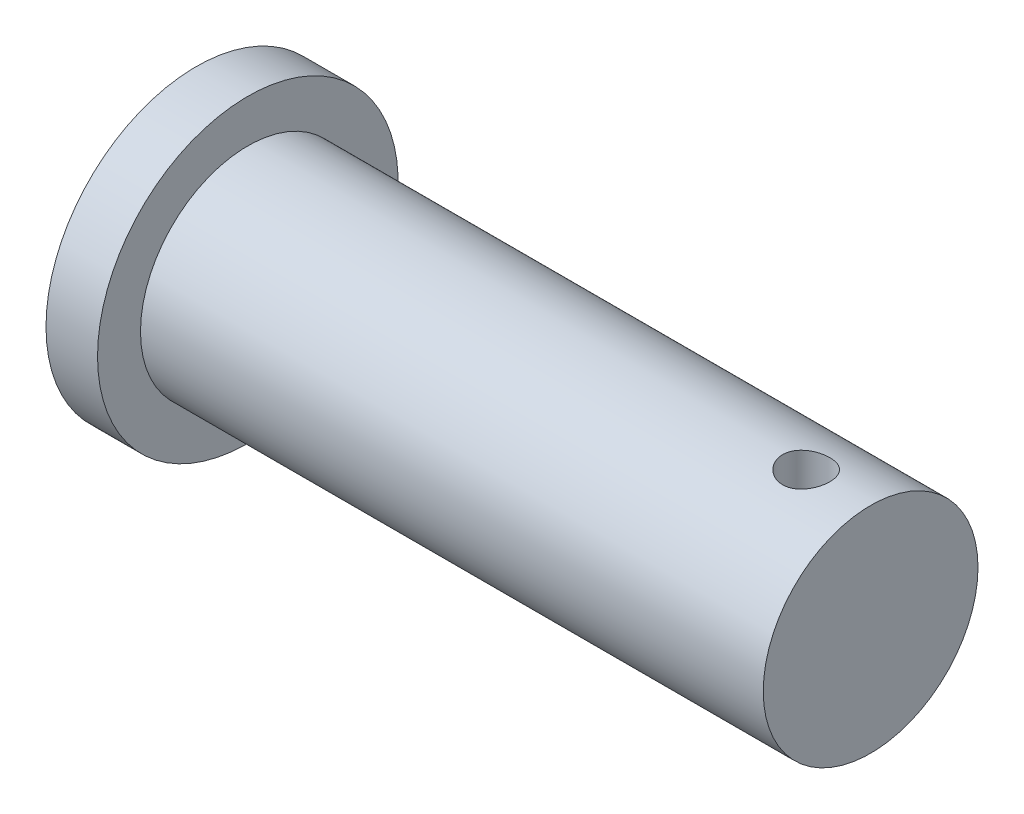
ISO-10303-21;
HEADER;
FILE_DESCRIPTION(('STEP AP214'),'2;1');
FILE_NAME('part.step','',(''),(''),'','','');
FILE_SCHEMA(('AUTOMOTIVE_DESIGN { 1 0 10303 214 1 1 1 1 }'));
ENDSEC;
DATA;
#1=APPLICATION_CONTEXT('core data for automotive mechanical design processes');
#2=APPLICATION_PROTOCOL_DEFINITION('international standard','automotive_design',2000,#1);
#3=PRODUCT_CONTEXT('',#1,'mechanical');
#4=PRODUCT('Part','Part','',(#3));
#5=PRODUCT_RELATED_PRODUCT_CATEGORY('part','',(#4));
#6=PRODUCT_DEFINITION_FORMATION('','',#4);
#7=PRODUCT_DEFINITION_CONTEXT('part definition',#1,'design');
#8=PRODUCT_DEFINITION('design','',#6,#7);
#9=PRODUCT_DEFINITION_SHAPE('','',#8);
#10=(LENGTH_UNIT() NAMED_UNIT(*) SI_UNIT(.MILLI.,.METRE.));
#11=(NAMED_UNIT(*) PLANE_ANGLE_UNIT() SI_UNIT($,.RADIAN.));
#12=(NAMED_UNIT(*) SI_UNIT($,.STERADIAN.) SOLID_ANGLE_UNIT());
#13=UNCERTAINTY_MEASURE_WITH_UNIT(LENGTH_MEASURE(1.E-05),#10,'distance_accuracy_value','');
#14=(GEOMETRIC_REPRESENTATION_CONTEXT(3) GLOBAL_UNCERTAINTY_ASSIGNED_CONTEXT((#13)) GLOBAL_UNIT_ASSIGNED_CONTEXT((#10,
#11,#12)) REPRESENTATION_CONTEXT('',''));
#15=CARTESIAN_POINT('',(0.,0.,0.));
#16=DIRECTION('',(0.,0.,1.));
#17=DIRECTION('',(1.,0.,0.));
#18=AXIS2_PLACEMENT_3D('',#15,#16,#17);
#19=CARTESIAN_POINT('',(0.,0.,0.));
#20=DIRECTION('',(-1.,0.,0.));
#21=DIRECTION('',(0.,0.,1.));
#22=AXIS2_PLACEMENT_3D('',#19,#20,#21);
#23=PLANE('',#22);
#24=CARTESIAN_POINT('',(0.,0.,0.));
#25=DIRECTION('',(-1.,0.,0.));
#26=DIRECTION('',(0.,0.,1.));
#27=AXIS2_PLACEMENT_3D('',#24,#25,#26);
#28=CIRCLE('',#27,25.);
#29=CARTESIAN_POINT('',(0.,0.,25.));
#30=VERTEX_POINT('',#29);
#31=EDGE_CURVE('E10',#30,#30,#28,.T.);
#32=ORIENTED_EDGE('',*,*,#31,.F.);
#33=EDGE_LOOP('',(#32));
#34=FACE_BOUND('',#33,.T.);
#35=ADVANCED_FACE('F40',(#34),#23,.F.);
#36=CARTESIAN_POINT('',(-157.,0.,0.));
#37=DIRECTION('',(-1.,0.,0.));
#38=DIRECTION('',(0.,0.,1.));
#39=AXIS2_PLACEMENT_3D('',#36,#37,#38);
#40=CYLINDRICAL_SURFACE('',#39,25.);
#41=CARTESIAN_POINT('',(-15.,-24.3904417040044,5.48692568598891));
#42=CARTESIAN_POINT('',(-14.8478528641094,-24.3904395836903,5.48692924756694));
#43=CARTESIAN_POINT('',(-14.6957479571834,-24.3918678962501,5.48059592767505));
#44=CARTESIAN_POINT('',(-14.3925972176209,-24.3975336229078,5.45532193090576));
#45=CARTESIAN_POINT('',(-14.2415515466732,-24.4017714568271,5.43637936985256));
#46=CARTESIAN_POINT('',(-13.9415915337901,-24.4129348837435,5.38602539426889));
#47=CARTESIAN_POINT('',(-13.7926781776191,-24.4198616807326,5.3546083941232));
#48=CARTESIAN_POINT('',(-13.4980468524885,-24.4361999383677,5.27954615966004));
#49=CARTESIAN_POINT('',(-13.3523300831978,-24.4456123151325,5.23589641631378));
#50=CARTESIAN_POINT('',(-13.0653791092844,-24.4666294394848,5.13678918348664));
#51=CARTESIAN_POINT('',(-12.9241385439275,-24.4782308966807,5.08134939984436));
#52=CARTESIAN_POINT('',(-12.6468185378473,-24.503306515237,4.95901875904935));
#53=CARTESIAN_POINT('',(-12.5107410248712,-24.516781367483,4.89212367519975));
#54=CARTESIAN_POINT('',(-12.2447601676808,-24.5452136370017,4.7474119047192));
#55=CARTESIAN_POINT('',(-12.1148543126789,-24.5601704436025,4.66959971126952));
#56=CARTESIAN_POINT('',(-11.8619562741839,-24.5911611433349,4.50354605402883));
#57=CARTESIAN_POINT('',(-11.7389667046449,-24.6071954387357,4.41530068567846));
#58=CARTESIAN_POINT('',(-11.4989687085544,-24.64014053352,4.22760979246244));
#59=CARTESIAN_POINT('',(-11.3820768582968,-24.6570608393303,4.12801684130962));
#60=CARTESIAN_POINT('',(-11.157020377272,-24.6910866043479,3.91936434001354));
#61=CARTESIAN_POINT('',(-11.0488589990536,-24.708192129892,3.81030129289663));
#62=CARTESIAN_POINT('',(-10.8420656665572,-24.7421030045069,3.5835009196093));
#63=CARTESIAN_POINT('',(-10.743430985574,-24.7589084383399,3.46576609255823));
#64=CARTESIAN_POINT('',(-10.5562953996071,-24.7917660983009,3.22233176595538));
#65=CARTESIAN_POINT('',(-10.4677982416418,-24.8078180446402,3.09662934792782));
#66=CARTESIAN_POINT('',(-10.3007488709965,-24.8388767869822,2.8368092804834));
#67=CARTESIAN_POINT('',(-10.2223078965471,-24.8538711831744,2.70261857916762));
#68=CARTESIAN_POINT('',(-10.0770014061407,-24.8822121574982,2.42787983092134));
#69=CARTESIAN_POINT('',(-10.0101402446399,-24.8955581152147,2.28732941744326));
#70=CARTESIAN_POINT('',(-9.88857184618348,-24.9202085006058,2.00095654889405));
#71=CARTESIAN_POINT('',(-9.83385903768034,-24.9315138637027,1.85513654642008));
#72=CARTESIAN_POINT('',(-9.73696961589609,-24.9517719248448,1.55921536766027));
#73=CARTESIAN_POINT('',(-9.6947975366843,-24.9607237718468,1.40911266441828));
#74=CARTESIAN_POINT('',(-9.5888423449196,-24.9833807245014,0.958910130029007));
#75=CARTESIAN_POINT('',(-9.54355196513864,-24.9933206851496,0.654019410500791));
#76=CARTESIAN_POINT('',(-9.50462705939392,-25.0018487688896,0.0409850693789847));
#77=CARTESIAN_POINT('',(-9.51098658498408,-25.000438199206,-0.267158173543922));
#78=CARTESIAN_POINT('',(-9.57450705524629,-24.986570452242,-0.87257594471877));
#79=CARTESIAN_POINT('',(-9.63079579672567,-24.9743029409154,-1.16994623411821));
#80=CARTESIAN_POINT('',(-9.79120550636413,-24.9403105756923,-1.75090253049288));
#81=CARTESIAN_POINT('',(-9.89532864699154,-24.9185852922599,-2.03448791075962));
#82=CARTESIAN_POINT('',(-10.1492167350271,-24.8678150883284,-2.58225793847721));
#83=CARTESIAN_POINT('',(-10.2993119276261,-24.8387174782121,-2.84628445524353));
#84=CARTESIAN_POINT('',(-10.6406384387953,-24.7763919690909,-3.34571962900131));
#85=CARTESIAN_POINT('',(-10.8318753972202,-24.743163504078,-3.58112435548765));
#86=CARTESIAN_POINT('',(-11.254804822667,-24.6754079178853,-4.02182398901012));
#87=CARTESIAN_POINT('',(-11.4872608508519,-24.6408681737786,-4.22638483396158));
#88=CARTESIAN_POINT('',(-11.9835354351618,-24.5750346143725,-4.59375761361559));
#89=CARTESIAN_POINT('',(-12.2473548529753,-24.5437408882996,-4.75656840087455));
#90=CARTESIAN_POINT('',(-12.800059856081,-24.4879089633101,-5.03614897541112));
#91=CARTESIAN_POINT('',(-13.0890182640809,-24.4633913121985,-5.15277917723493));
#92=CARTESIAN_POINT('',(-13.6830984979499,-24.4241716892725,-5.33560409890557));
#93=CARTESIAN_POINT('',(-13.9882177319601,-24.4094681485938,-5.40180688021895));
#94=CARTESIAN_POINT('',(-14.5992486549309,-24.3918617187914,-5.4807573019737));
#95=CARTESIAN_POINT('',(-14.9050155510316,-24.3887228252692,-5.49457417546741));
#96=CARTESIAN_POINT('',(-15.514483821339,-24.3939643269164,-5.4712561265428));
#97=CARTESIAN_POINT('',(-15.8181853370327,-24.4023439248678,-5.43412473035613));
#98=CARTESIAN_POINT('',(-16.4111732550927,-24.4294552991797,-5.31089210736716));
#99=CARTESIAN_POINT('',(-16.7005884315407,-24.4480623430502,-5.22538055668244));
#100=CARTESIAN_POINT('',(-17.2609831892765,-24.4934194067747,-5.00845373119411));
#101=CARTESIAN_POINT('',(-17.5319609929918,-24.5201702104226,-4.87703403779463));
#102=CARTESIAN_POINT('',(-18.0524138949794,-24.5793186897184,-4.56966870641581));
#103=CARTESIAN_POINT('',(-18.3014908613144,-24.6117974227195,-4.39306484490186));
#104=CARTESIAN_POINT('',(-18.7668659139383,-24.678528743473,-4.0012038210895));
#105=CARTESIAN_POINT('',(-18.983159893981,-24.7127815527183,-3.78594182401648));
#106=CARTESIAN_POINT('',(-19.3809837935675,-24.7799802319991,-3.31803920808596));
#107=CARTESIAN_POINT('',(-19.561784499393,-24.8128894735023,-3.06477249794606));
#108=CARTESIAN_POINT('',(-19.8782718213509,-24.8730164701174,-2.53082850634251));
#109=CARTESIAN_POINT('',(-20.0139605520525,-24.9002344919761,-2.25015251045399));
#110=CARTESIAN_POINT('',(-20.2353630699165,-24.9457605411793,-1.67117157922903));
#111=CARTESIAN_POINT('',(-20.3213946539106,-24.9641251014865,-1.37299251377133));
#112=CARTESIAN_POINT('',(-20.4420164361445,-24.9901099983033,-0.765791181035985));
#113=CARTESIAN_POINT('',(-20.4766141666779,-24.997731908025,-0.456770508256938));
#114=CARTESIAN_POINT('',(-20.4890304889155,-25.0004644930119,0.00429168299274479));
#115=CARTESIAN_POINT('',(-20.4868059851242,-24.9999730894024,0.156027971773244));
#116=CARTESIAN_POINT('',(-20.4698114592478,-24.9962472869036,0.458746902649513));
#117=CARTESIAN_POINT('',(-20.4550462284491,-24.9930139355982,0.609729810423857));
#118=CARTESIAN_POINT('',(-20.4130765404903,-24.9838875149462,0.909915354030994));
#119=CARTESIAN_POINT('',(-20.3858678547478,-24.9779935414655,1.05911736697342));
#120=CARTESIAN_POINT('',(-20.3192435072261,-24.9637124299868,1.35459443600505));
#121=CARTESIAN_POINT('',(-20.2798321905096,-24.955326179471,1.50087051424282));
#122=CARTESIAN_POINT('',(-20.1892399193818,-24.9363169772317,1.78910566770361));
#123=CARTESIAN_POINT('',(-20.1380938302124,-24.9257006590113,1.93107614804683));
#124=CARTESIAN_POINT('',(-20.0243743675087,-24.9025076765705,2.21013793327368));
#125=CARTESIAN_POINT('',(-19.9618050161174,-24.8899317025745,2.3472309352854));
#126=CARTESIAN_POINT('',(-19.8256530377953,-24.863147812645,2.61573982644339));
#127=CARTESIAN_POINT('',(-19.7520657529898,-24.8489392071038,2.74715328411512));
#128=CARTESIAN_POINT('',(-19.5944415261934,-24.8192778374394,3.00334370453694));
#129=CARTESIAN_POINT('',(-19.5104081232546,-24.8038254953052,3.12812289457408));
#130=CARTESIAN_POINT('',(-19.3307074244298,-24.7717724071377,3.37265385451534));
#131=CARTESIAN_POINT('',(-19.2348455053337,-24.7551551615408,3.49226047842446));
#132=CARTESIAN_POINT('',(-19.0335239236439,-24.7215112487739,3.7229651537068));
#133=CARTESIAN_POINT('',(-18.9280676054197,-24.7044847257789,3.83406614525374));
#134=CARTESIAN_POINT('',(-18.708167998545,-24.6704753275265,4.04713425462087));
#135=CARTESIAN_POINT('',(-18.593719362796,-24.6534924845358,4.14909585956662));
#136=CARTESIAN_POINT('',(-18.3566924988134,-24.6200583425484,4.34308812872971));
#137=CARTESIAN_POINT('',(-18.2341172589599,-24.6036068514322,4.43512241115472));
#138=CARTESIAN_POINT('',(-17.9798523335412,-24.5714681487794,4.60987622477299));
#139=CARTESIAN_POINT('',(-17.8480596715423,-24.5557947325587,4.69244856471365));
#140=CARTESIAN_POINT('',(-17.5778651974749,-24.5259253549593,4.8461442692415));
#141=CARTESIAN_POINT('',(-17.4394658441793,-24.5117288500855,4.91727185074093));
#142=CARTESIAN_POINT('',(-17.1570460728126,-24.485235421675,5.04754084924169));
#143=CARTESIAN_POINT('',(-17.0130287955984,-24.4729374552467,5.10668885239123));
#144=CARTESIAN_POINT('',(-16.7203803945664,-24.4506042221252,5.2125683761294));
#145=CARTESIAN_POINT('',(-16.5717501011193,-24.4405685508621,5.25930211704843));
#146=CARTESIAN_POINT('',(-16.1901478617738,-24.4183741072347,5.36163339211002));
#147=CARTESIAN_POINT('',(-15.9546844269499,-24.4079622588575,5.40854739445524));
#148=CARTESIAN_POINT('',(-15.479445589671,-24.3939978966866,5.47118996590937));
#149=CARTESIAN_POINT('',(-15.2396704008206,-24.3904450440377,5.48692007559848));
#150=CARTESIAN_POINT('',(-15.,-24.3904417040044,5.48692568598891));
#151=B_SPLINE_CURVE_WITH_KNOTS('',3,(#41,#42,#43,#44,#45,#46,#47,#48,#49,#50,#51,#52,#53,#54,
#55,#56,#57,#58,#59,#60,#61,#62,#63,#64,#65,#66,#67,#68,#69,#70,#71,#72,#73,#74,#75,#76,#77,#78,
#79,#80,#81,#82,#83,#84,#85,#86,#87,#88,#89,#90,#91,#92,#93,#94,#95,#96,#97,#98,#99,#100,#101,
#102,#103,#104,#105,#106,#107,#108,#109,#110,#111,#112,#113,#114,#115,#116,#117,#118,#119,#120,
#121,#122,#123,#124,#125,#126,#127,#128,#129,#130,#131,#132,#133,#134,#135,#136,#137,#138,#139,
#140,#141,#142,#143,#144,#145,#146,#147,#148,#149,#150),.UNSPECIFIED.,.T.,.F.,(4,2,2,2,2,2,2,2,
2,2,2,2,2,2,2,2,2,2,2,2,2,2,2,2,2,2,2,2,2,2,2,2,2,2,2,2,2,2,2,2,2,2,2,2,2,2,2,2,2,2,2,2,2,2,4),
(0.,0.456230363003332,0.912528914982533,1.36903201223289,1.82570359982593,2.2816941580224,
2.73785332839557,3.1938253039914,3.64996846804038,4.1129153679468,4.5760339508434,
5.0390195859565,5.50217580079963,5.97007955624501,6.43815888131014,6.90602308768261,
7.37405624410114,8.29433341879706,9.21450460798402,10.1189113030548,11.0233590771232,
11.9344628035656,12.8456915069147,13.7760091213121,14.7063523014849,15.6394864549394,
16.5724714036684,17.4863076471811,18.4000806454495,19.3029490086374,20.205904295623,
21.1228474650261,22.0399053917686,22.9741869554003,23.9084247195393,24.8366152722326,
25.7646698815284,26.2194851510891,26.6741267329174,27.1289229277204,27.5835573664416,
28.0368581403902,28.4899996133866,28.9433331974566,29.3965136125891,29.8585156496311,
30.3203572567737,30.782475597789,31.2444249375025,31.7127928154749,32.1809877224324,
32.6489245216514,33.1167775724461,33.8354918335068,34.5541705869877),.UNSPECIFIED.);
#152=CARTESIAN_POINT('',(-15.,-24.3904417040044,5.48692568598891));
#153=VERTEX_POINT('',#152);
#154=EDGE_CURVE('E37',#153,#153,#151,.T.);
#155=ORIENTED_EDGE('',*,*,#154,.T.);
#156=EDGE_LOOP('',(#155));
#157=FACE_BOUND('',#156,.T.);
#158=CARTESIAN_POINT('',(-15.,24.3904417040044,5.48692568598891));
#159=CARTESIAN_POINT('',(-15.1521471358906,24.3904395836903,5.48692924756694));
#160=CARTESIAN_POINT('',(-15.3042520428165,24.3918678962501,5.48059592767505));
#161=CARTESIAN_POINT('',(-15.6074027823791,24.3975336229078,5.45532193090576));
#162=CARTESIAN_POINT('',(-15.7584484533268,24.4017714568271,5.43637936985256));
#163=CARTESIAN_POINT('',(-16.0584084662099,24.4129348837435,5.38602539426889));
#164=CARTESIAN_POINT('',(-16.2073218223809,24.4198616807326,5.3546083941232));
#165=CARTESIAN_POINT('',(-16.5019531475114,24.4361999383677,5.27954615966004));
#166=CARTESIAN_POINT('',(-16.6476699168022,24.4456123151325,5.23589641631378));
#167=CARTESIAN_POINT('',(-16.9346208907156,24.4666294394848,5.13678918348664));
#168=CARTESIAN_POINT('',(-17.0758614560725,24.4782308966807,5.08134939984436));
#169=CARTESIAN_POINT('',(-17.3531814621527,24.503306515237,4.95901875904935));
#170=CARTESIAN_POINT('',(-17.4892589751288,24.516781367483,4.89212367519975));
#171=CARTESIAN_POINT('',(-17.7552398323192,24.5452136370017,4.7474119047192));
#172=CARTESIAN_POINT('',(-17.885145687321,24.5601704436025,4.66959971126953));
#173=CARTESIAN_POINT('',(-18.138043725816,24.5911611433349,4.50354605402883));
#174=CARTESIAN_POINT('',(-18.261033295355,24.6071954387357,4.41530068567846));
#175=CARTESIAN_POINT('',(-18.5010312914456,24.64014053352,4.22760979246244));
#176=CARTESIAN_POINT('',(-18.6179231417032,24.6570608393303,4.12801684130962));
#177=CARTESIAN_POINT('',(-18.842979622728,24.6910866043479,3.91936434001354));
#178=CARTESIAN_POINT('',(-18.9511410009463,24.708192129892,3.81030129289663));
#179=CARTESIAN_POINT('',(-19.1579343334428,24.7421030045069,3.58350091960931));
#180=CARTESIAN_POINT('',(-19.2565690144259,24.7589084383399,3.46576609255824));
#181=CARTESIAN_POINT('',(-19.4437046003928,24.7917660983009,3.22233176595538));
#182=CARTESIAN_POINT('',(-19.5322017583582,24.8078180446402,3.09662934792783));
#183=CARTESIAN_POINT('',(-19.6992511290035,24.8388767869822,2.83680928048341));
#184=CARTESIAN_POINT('',(-19.7776921034529,24.8538711831744,2.70261857916762));
#185=CARTESIAN_POINT('',(-19.9229985938593,24.8822121574982,2.42787983092134));
#186=CARTESIAN_POINT('',(-19.9898597553601,24.8955581152147,2.28732941744327));
#187=CARTESIAN_POINT('',(-20.1114281538165,24.9202085006058,2.00095654889405));
#188=CARTESIAN_POINT('',(-20.1661409623196,24.9315138637027,1.85513654642009));
#189=CARTESIAN_POINT('',(-20.2630303841039,24.9517719248448,1.55921536766027));
#190=CARTESIAN_POINT('',(-20.3052024633157,24.9607237718468,1.40911266441829));
#191=CARTESIAN_POINT('',(-20.4111576550804,24.9833807245014,0.95891013002901));
#192=CARTESIAN_POINT('',(-20.4564480348613,24.9933206851496,0.654019410500793));
#193=CARTESIAN_POINT('',(-20.4953729406061,25.0018487688896,0.0409850693789873));
#194=CARTESIAN_POINT('',(-20.4890134150159,25.000438199206,-0.267158173543919));
#195=CARTESIAN_POINT('',(-20.4254929447537,24.986570452242,-0.872575944718767));
#196=CARTESIAN_POINT('',(-20.3692042032743,24.9743029409154,-1.16994623411821));
#197=CARTESIAN_POINT('',(-20.2087944936358,24.9403105756923,-1.75090253049288));
#198=CARTESIAN_POINT('',(-20.1046713530084,24.9185852922599,-2.03448791075962));
#199=CARTESIAN_POINT('',(-19.8507832649729,24.8678150883284,-2.58225793847721));
#200=CARTESIAN_POINT('',(-19.7006880723739,24.8387174782121,-2.84628445524353));
#201=CARTESIAN_POINT('',(-19.3593615612047,24.7763919690909,-3.34571962900131));
#202=CARTESIAN_POINT('',(-19.1681246027798,24.743163504078,-3.58112435548765));
#203=CARTESIAN_POINT('',(-18.745195177333,24.6754079178853,-4.02182398901012));
#204=CARTESIAN_POINT('',(-18.512739149148,24.6408681737786,-4.22638483396158));
#205=CARTESIAN_POINT('',(-18.0164645648382,24.5750346143725,-4.59375761361559));
#206=CARTESIAN_POINT('',(-17.7526451470247,24.5437408882996,-4.75656840087455));
#207=CARTESIAN_POINT('',(-17.199940143919,24.4879089633101,-5.03614897541112));
#208=CARTESIAN_POINT('',(-16.9109817359191,24.4633913121985,-5.15277917723493));
#209=CARTESIAN_POINT('',(-16.3169015020501,24.4241716892725,-5.33560409890557));
#210=CARTESIAN_POINT('',(-16.0117822680399,24.4094681485938,-5.40180688021895));
#211=CARTESIAN_POINT('',(-15.4007513450691,24.3918617187914,-5.4807573019737));
#212=CARTESIAN_POINT('',(-15.0949844489683,24.3887228252692,-5.49457417546741));
#213=CARTESIAN_POINT('',(-14.485516178661,24.3939643269164,-5.4712561265428));
#214=CARTESIAN_POINT('',(-14.1818146629673,24.4023439248678,-5.43412473035613));
#215=CARTESIAN_POINT('',(-13.5888267449072,24.4294552991797,-5.31089210736716));
#216=CARTESIAN_POINT('',(-13.2994115684592,24.4480623430502,-5.22538055668244));
#217=CARTESIAN_POINT('',(-12.7390168107235,24.4934194067747,-5.00845373119411));
#218=CARTESIAN_POINT('',(-12.4680390070081,24.5201702104226,-4.87703403779463));
#219=CARTESIAN_POINT('',(-11.9475861050206,24.5793186897184,-4.56966870641581));
#220=CARTESIAN_POINT('',(-11.6985091386856,24.6117974227195,-4.39306484490185));
#221=CARTESIAN_POINT('',(-11.2331340860617,24.678528743473,-4.0012038210895));
#222=CARTESIAN_POINT('',(-11.016840106019,24.7127815527183,-3.78594182401648));
#223=CARTESIAN_POINT('',(-10.6190162064325,24.7799802319991,-3.31803920808597));
#224=CARTESIAN_POINT('',(-10.438215500607,24.8128894735023,-3.06477249794607));
#225=CARTESIAN_POINT('',(-10.121728178649,24.8730164701174,-2.53082850634251));
#226=CARTESIAN_POINT('',(-9.98603944794751,24.9002344919761,-2.250152510454));
#227=CARTESIAN_POINT('',(-9.76463693008352,24.9457605411793,-1.67117157922903));
#228=CARTESIAN_POINT('',(-9.67860534608938,24.9641251014865,-1.37299251377134));
#229=CARTESIAN_POINT('',(-9.55798356385551,24.9901099983033,-0.765791181035986));
#230=CARTESIAN_POINT('',(-9.52338583332209,24.997731908025,-0.456770508256939));
#231=CARTESIAN_POINT('',(-9.51096951108448,25.0004644930119,0.00429168299274408));
#232=CARTESIAN_POINT('',(-9.51319401487579,24.9999730894024,0.156027971773243));
#233=CARTESIAN_POINT('',(-9.53018854075213,24.9962472869036,0.458746902649513));
#234=CARTESIAN_POINT('',(-9.54495377155084,24.9930139355982,0.609729810423857));
#235=CARTESIAN_POINT('',(-9.58692345950963,24.9838875149462,0.909915354030994));
#236=CARTESIAN_POINT('',(-9.61413214525221,24.9779935414655,1.05911736697342));
#237=CARTESIAN_POINT('',(-9.68075649277392,24.9637124299868,1.35459443600505));
#238=CARTESIAN_POINT('',(-9.72016780949038,24.955326179471,1.50087051424282));
#239=CARTESIAN_POINT('',(-9.81076008061816,24.9363169772317,1.78910566770361));
#240=CARTESIAN_POINT('',(-9.86190616978758,24.9257006590113,1.93107614804683));
#241=CARTESIAN_POINT('',(-9.97562563249128,24.9025076765705,2.21013793327368));
#242=CARTESIAN_POINT('',(-10.0381949838825,24.8899317025745,2.3472309352854));
#243=CARTESIAN_POINT('',(-10.1743469622047,24.863147812645,2.61573982644339));
#244=CARTESIAN_POINT('',(-10.2479342470102,24.8489392071038,2.74715328411512));
#245=CARTESIAN_POINT('',(-10.4055584738066,24.8192778374394,3.00334370453694));
#246=CARTESIAN_POINT('',(-10.4895918767454,24.8038254953052,3.12812289457408));
#247=CARTESIAN_POINT('',(-10.6692925755701,24.7717724071377,3.37265385451534));
#248=CARTESIAN_POINT('',(-10.7651544946663,24.7551551615408,3.49226047842446));
#249=CARTESIAN_POINT('',(-10.966476076356,24.7215112487739,3.72296515370679));
#250=CARTESIAN_POINT('',(-11.0719323945803,24.7044847257789,3.83406614525374));
#251=CARTESIAN_POINT('',(-11.291832001455,24.6704753275265,4.04713425462087));
#252=CARTESIAN_POINT('',(-11.4062806372039,24.6534924845358,4.14909585956662));
#253=CARTESIAN_POINT('',(-11.6433075011865,24.6200583425484,4.34308812872971));
#254=CARTESIAN_POINT('',(-11.7658827410401,24.6036068514322,4.43512241115472));
#255=CARTESIAN_POINT('',(-12.0201476664588,24.5714681487794,4.60987622477299));
#256=CARTESIAN_POINT('',(-12.1519403284577,24.5557947325587,4.69244856471365));
#257=CARTESIAN_POINT('',(-12.422134802525,24.5259253549593,4.84614426924151));
#258=CARTESIAN_POINT('',(-12.5605341558207,24.5117288500855,4.91727185074093));
#259=CARTESIAN_POINT('',(-12.8429539271874,24.485235421675,5.04754084924169));
#260=CARTESIAN_POINT('',(-12.9869712044015,24.4729374552467,5.10668885239123));
#261=CARTESIAN_POINT('',(-13.2796196054336,24.4506042221252,5.2125683761294));
#262=CARTESIAN_POINT('',(-13.4282498988807,24.4405685508621,5.25930211704843));
#263=CARTESIAN_POINT('',(-13.8098521382261,24.4183741072347,5.36163339211002));
#264=CARTESIAN_POINT('',(-14.0453155730501,24.4079622588575,5.40854739445524));
#265=CARTESIAN_POINT('',(-14.520554410329,24.3939978966866,5.47118996590937));
#266=CARTESIAN_POINT('',(-14.7603295991794,24.3904450440377,5.48692007559848));
#267=CARTESIAN_POINT('',(-15.,24.3904417040044,5.48692568598891));
#268=B_SPLINE_CURVE_WITH_KNOTS('',3,(#158,#159,#160,#161,#162,#163,#164,#165,#166,#167,#168,
#169,#170,#171,#172,#173,#174,#175,#176,#177,#178,#179,#180,#181,#182,#183,#184,#185,#186,#187,
#188,#189,#190,#191,#192,#193,#194,#195,#196,#197,#198,#199,#200,#201,#202,#203,#204,#205,#206,
#207,#208,#209,#210,#211,#212,#213,#214,#215,#216,#217,#218,#219,#220,#221,#222,#223,#224,#225,
#226,#227,#228,#229,#230,#231,#232,#233,#234,#235,#236,#237,#238,#239,#240,#241,#242,#243,#244,
#245,#246,#247,#248,#249,#250,#251,#252,#253,#254,#255,#256,#257,#258,#259,#260,#261,#262,#263,
#264,#265,#266,#267),.UNSPECIFIED.,.T.,.F.,(4,2,2,2,2,2,2,2,2,2,2,2,2,2,2,2,2,2,2,2,2,2,2,2,2,2,
2,2,2,2,2,2,2,2,2,2,2,2,2,2,2,2,2,2,2,2,2,2,2,2,2,2,2,2,4),(0.,0.45623036300333,
0.912528914982531,1.36903201223289,1.82570359982592,2.2816941580224,2.73785332839556,
3.1938253039914,3.64996846804038,4.1129153679468,4.5760339508434,5.03901958595649,
5.50217580079962,5.97007955624501,6.43815888131014,6.9060230876826,7.37405624410114,
8.29433341879706,9.21450460798402,10.1189113030548,11.0233590771232,11.9344628035656,
12.8456915069147,13.7760091213121,14.7063523014849,15.6394864549394,16.5724714036684,
17.4863076471811,18.4000806454495,19.3029490086374,20.205904295623,21.1228474650261,
22.0399053917686,22.9741869554003,23.9084247195393,24.8366152722326,25.7646698815284,
26.2194851510891,26.6741267329174,27.1289229277204,27.5835573664416,28.0368581403902,
28.4899996133866,28.9433331974566,29.3965136125891,29.8585156496311,30.3203572567737,
30.782475597789,31.2444249375025,31.7127928154749,32.1809877224324,32.6489245216514,
33.1167775724461,33.8354918335068,34.5541705869877),.UNSPECIFIED.);
#269=CARTESIAN_POINT('',(-15.,24.3904417040044,5.48692568598891));
#270=VERTEX_POINT('',#269);
#271=EDGE_CURVE('E57',#270,#270,#268,.T.);
#272=ORIENTED_EDGE('',*,*,#271,.T.);
#273=EDGE_LOOP('',(#272));
#274=FACE_BOUND('',#273,.T.);
#275=CARTESIAN_POINT('',(-145.,0.,0.));
#276=DIRECTION('',(-1.,0.,0.));
#277=DIRECTION('',(0.,0.,1.));
#278=AXIS2_PLACEMENT_3D('',#275,#276,#277);
#279=CIRCLE('',#278,25.);
#280=CARTESIAN_POINT('',(-145.,0.,25.));
#281=VERTEX_POINT('',#280);
#282=EDGE_CURVE('E48',#281,#281,#279,.T.);
#283=ORIENTED_EDGE('',*,*,#282,.F.);
#284=EDGE_LOOP('',(#283));
#285=FACE_BOUND('',#284,.T.);
#286=ORIENTED_EDGE('',*,*,#31,.T.);
#287=EDGE_LOOP('',(#286));
#288=FACE_BOUND('',#287,.T.);
#289=ADVANCED_FACE('F64',(#157,#274,#285,#288),#40,.T.);
#290=CARTESIAN_POINT('',(-145.,25.,0.));
#291=DIRECTION('',(-1.,0.,0.));
#292=DIRECTION('',(0.,0.,1.));
#293=AXIS2_PLACEMENT_3D('',#290,#291,#292);
#294=PLANE('',#293);
#295=CARTESIAN_POINT('',(-145.,0.,0.));
#296=DIRECTION('',(-1.,0.,0.));
#297=DIRECTION('',(0.,0.,1.));
#298=AXIS2_PLACEMENT_3D('',#295,#296,#297);
#299=CIRCLE('',#298,35.);
#300=CARTESIAN_POINT('',(-145.,0.,35.));
#301=VERTEX_POINT('',#300);
#302=EDGE_CURVE('E52',#301,#301,#299,.T.);
#303=ORIENTED_EDGE('',*,*,#302,.F.);
#304=EDGE_LOOP('',(#303));
#305=FACE_BOUND('',#304,.T.);
#306=ORIENTED_EDGE('',*,*,#282,.T.);
#307=EDGE_LOOP('',(#306));
#308=FACE_BOUND('',#307,.T.);
#309=ADVANCED_FACE('F79',(#305,#308),#294,.F.);
#310=CARTESIAN_POINT('',(-157.,0.,0.));
#311=DIRECTION('',(-1.,0.,0.));
#312=DIRECTION('',(0.,0.,1.));
#313=AXIS2_PLACEMENT_3D('',#310,#311,#312);
#314=CYLINDRICAL_SURFACE('',#313,35.);
#315=CARTESIAN_POINT('',(-157.,0.,0.));
#316=DIRECTION('',(-1.,0.,0.));
#317=DIRECTION('',(0.,0.,1.));
#318=AXIS2_PLACEMENT_3D('',#315,#316,#317);
#319=CIRCLE('',#318,35.);
#320=CARTESIAN_POINT('',(-157.,0.,35.));
#321=VERTEX_POINT('',#320);
#322=EDGE_CURVE('E127',#321,#321,#319,.T.);
#323=ORIENTED_EDGE('',*,*,#322,.F.);
#324=EDGE_LOOP('',(#323));
#325=FACE_BOUND('',#324,.T.);
#326=ORIENTED_EDGE('',*,*,#302,.T.);
#327=EDGE_LOOP('',(#326));
#328=FACE_BOUND('',#327,.T.);
#329=ADVANCED_FACE('F71',(#325,#328),#314,.T.);
#330=CARTESIAN_POINT('',(-157.,35.,0.));
#331=DIRECTION('',(1.,0.,0.));
#332=DIRECTION('',(0.,0.,-1.));
#333=AXIS2_PLACEMENT_3D('',#330,#331,#332);
#334=PLANE('',#333);
#335=ORIENTED_EDGE('',*,*,#322,.T.);
#336=EDGE_LOOP('',(#335));
#337=FACE_BOUND('',#336,.T.);
#338=ADVANCED_FACE('F69',(#337),#334,.F.);
#339=CARTESIAN_POINT('',(-15.,-30.,0.));
#340=DIRECTION('',(0.,1.,0.));
#341=DIRECTION('',(0.,0.,1.));
#342=AXIS2_PLACEMENT_3D('',#339,#340,#341);
#343=CYLINDRICAL_SURFACE('',#342,5.48692568598891);
#344=ORIENTED_EDGE('',*,*,#271,.F.);
#345=EDGE_LOOP('',(#344));
#346=FACE_BOUND('',#345,.T.);
#347=ORIENTED_EDGE('',*,*,#154,.F.);
#348=EDGE_LOOP('',(#347));
#349=FACE_BOUND('',#348,.T.);
#350=ADVANCED_FACE('F63',(#346,#349),#343,.F.);
#351=CLOSED_SHELL('',(#35,#289,#309,#329,#338,#350));
#352=MANIFOLD_SOLID_BREP('B2',#351);
#353=ADVANCED_BREP_SHAPE_REPRESENTATION('',(#18,#352),#14);
#354=SHAPE_DEFINITION_REPRESENTATION(#9,#353);
ENDSEC;
END-ISO-10303-21;
